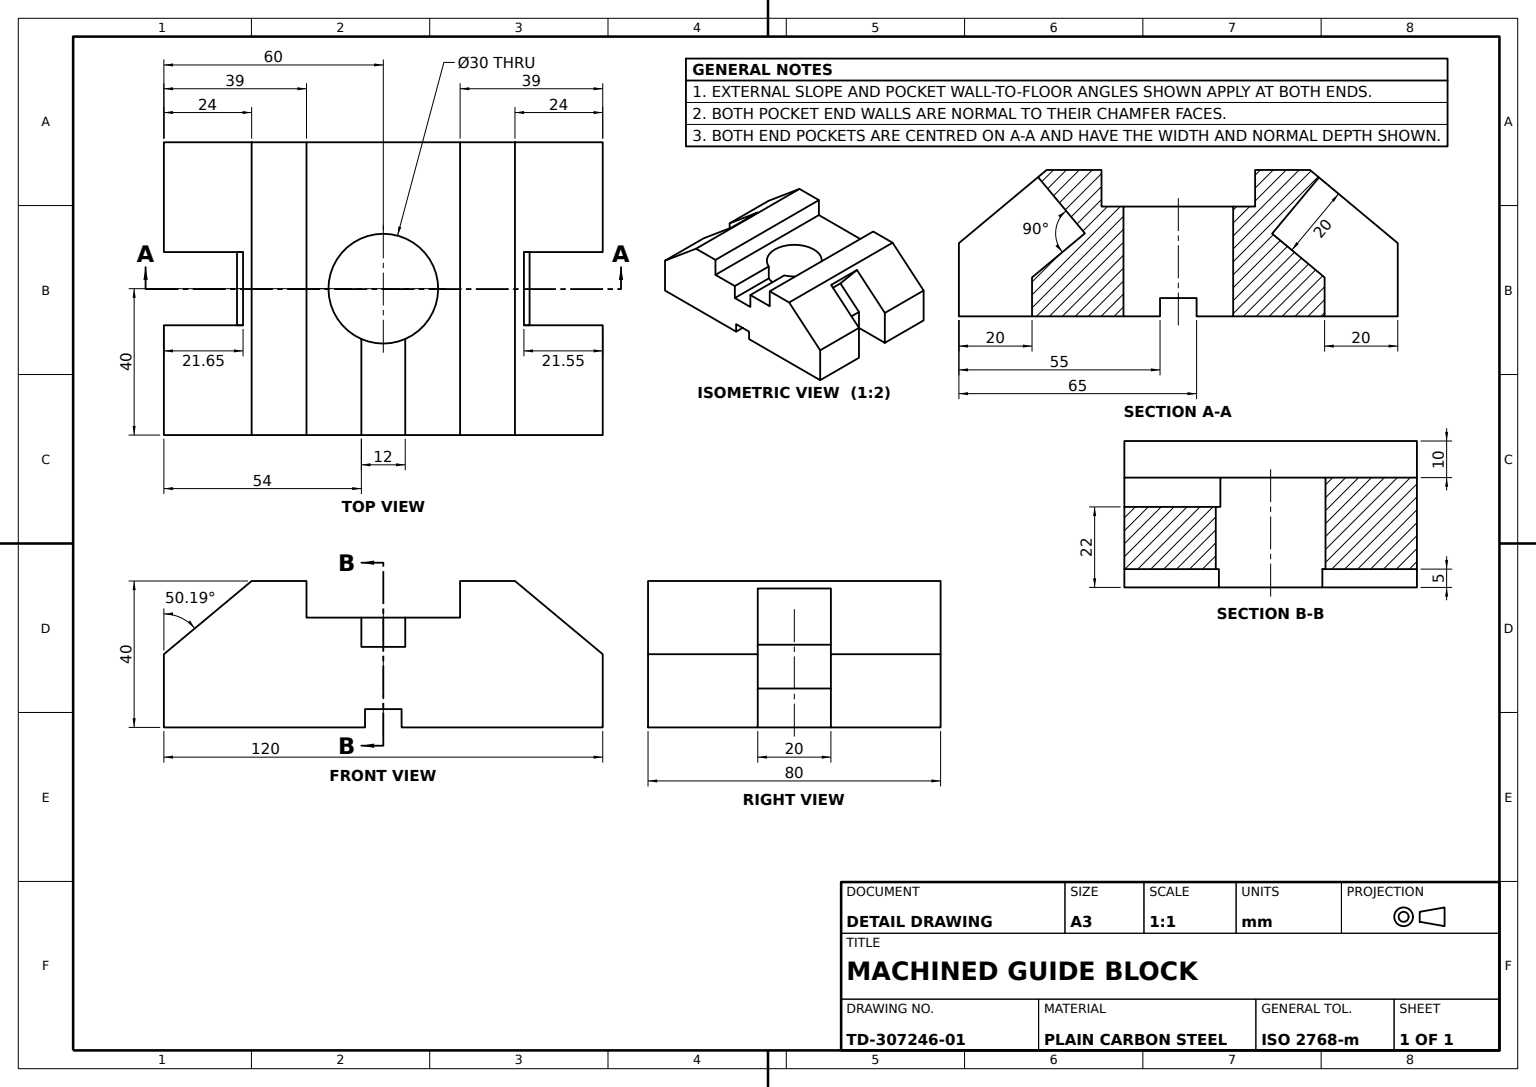
from build123d import *

# Parameters (mm, degrees)
BLOCK_BODY_EXTRUDE_80_DEPTH     = 80
THROUGH_CUT_SKETCH_R            = 15
THROUGH_CUT_80_DEPTH            = 80
PROFILE_CUT_30_DEPTH            = 30
POCKET_A_SKETCH_30X30_W         = 20
POCKET_A_SKETCH_30X30_H         = 20
SQUARE_POCKET_A_30X30X20_DEPTH  = 20
POCKET_A_EXTENSION_SKETCH_W     = 28.050217784
POCKET_A_EXTENSION_SKETCH_H     = 20
POCKET_A_EXTENSION_CUT_20_DEPTH = 20
POCKET_B_SKETCH_30X30_W         = 20
POCKET_B_SKETCH_30X30_H         = 20
SQUARE_POCKET_B_30X30X20_DEPTH  = 20
POCKET_B_EXTENSION_SKETCH_W     = 28.181918945
POCKET_B_EXTENSION_SKETCH_H     = 20
POCKET_B_EXTENSION_CUT_20_DEPTH = 20


with BuildPart() as part:
    # Block Profile Sketch → Block Body Extrude 80 (new body)
    with BuildSketch(Plane.XY):
        Polygon((0, 0), (0, 20), (24, 40), (39, 40), (39, 30), (54, 30), (66, 30), (81, 30), (81, 40), (96, 40), (120, 20), (120, 0), (65, 0), (65, 5), (55, 5), (55, 0), align=None)
    extrude(amount=BLOCK_BODY_EXTRUDE_80_DEPTH)

    # Through Cut Sketch → Through Cut 80 (cut)
    with BuildSketch(Plane(origin=(0, 30, 0), x_dir=(1, 0, 0), z_dir=(0, 1, 0))):
        with Locations(Location((60, -40, 0), (0, 0, 270))):
            Circle(THROUGH_CUT_SKETCH_R)
    extrude(amount=-THROUGH_CUT_80_DEPTH, mode=Mode.SUBTRACT)

    # Profile Cut Sketch → Profile Cut 30 (cut)
    with BuildSketch(Plane.XY.offset(80)):
        Polygon((60, 30), (66, 30), (66, 22), (54, 22), (54, 30), align=None)
    extrude(amount=-PROFILE_CUT_30_DEPTH, mode=Mode.SUBTRACT)

    # Pocket A Sketch 30x30 → Square Pocket A 30x30x20 (cut)
    with BuildSketch(Plane(origin=(120, 0, 0), x_dir=(0, 0, -1), z_dir=(1, 0, 0))):
        with Locations((-40, 10)):
            Rectangle(POCKET_A_SKETCH_30X30_W, POCKET_A_SKETCH_30X30_H)
    extrude(amount=-SQUARE_POCKET_A_30X30X20_DEPTH, mode=Mode.SUBTRACT)

    # Pocket A Extension Sketch → Pocket A Extension Cut 20 (cut)
    with BuildSketch(Plane(origin=(59.016393443, 70.819672131, 0), x_dir=(0.7682212795973757, -0.6401843996644799, 0), z_dir=(0.6401843996644799, 0.7682212795973757, 0))):
        with Locations((65.357756666, -40)):
            Rectangle(POCKET_A_EXTENSION_SKETCH_W, POCKET_A_EXTENSION_SKETCH_H)
    extrude(amount=-POCKET_A_EXTENSION_CUT_20_DEPTH, mode=Mode.SUBTRACT)

    # Pocket B Sketch 30x30 → Square Pocket B 30x30x20 (cut)
    with BuildSketch(Plane.ZY):
        with Locations((40, 10)):
            Rectangle(POCKET_B_SKETCH_30X30_W, POCKET_B_SKETCH_30X30_H)
    extrude(amount=-SQUARE_POCKET_B_30X30X20_DEPTH, mode=Mode.SUBTRACT)

    # Pocket B Extension Sketch → Pocket B Extension Cut 20 (cut)
    with BuildSketch(Plane(origin=(-9.836065574, 11.803278689, 0), x_dir=(0.7682212795973757, 0.6401843996644802, 0), z_dir=(-0.64018439966448, 0.7682212795973756, 0))):
        with Locations((26.894647466, -40)):
            Rectangle(POCKET_B_EXTENSION_SKETCH_W, POCKET_B_EXTENSION_SKETCH_H)
    extrude(amount=-POCKET_B_EXTENSION_CUT_20_DEPTH, mode=Mode.SUBTRACT)


solid = part.part
